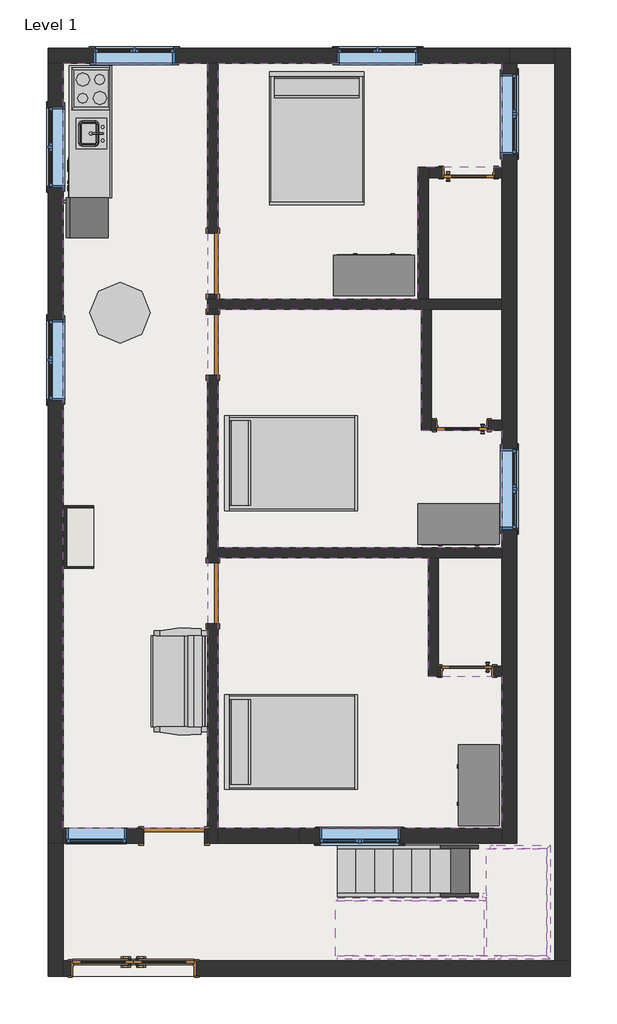
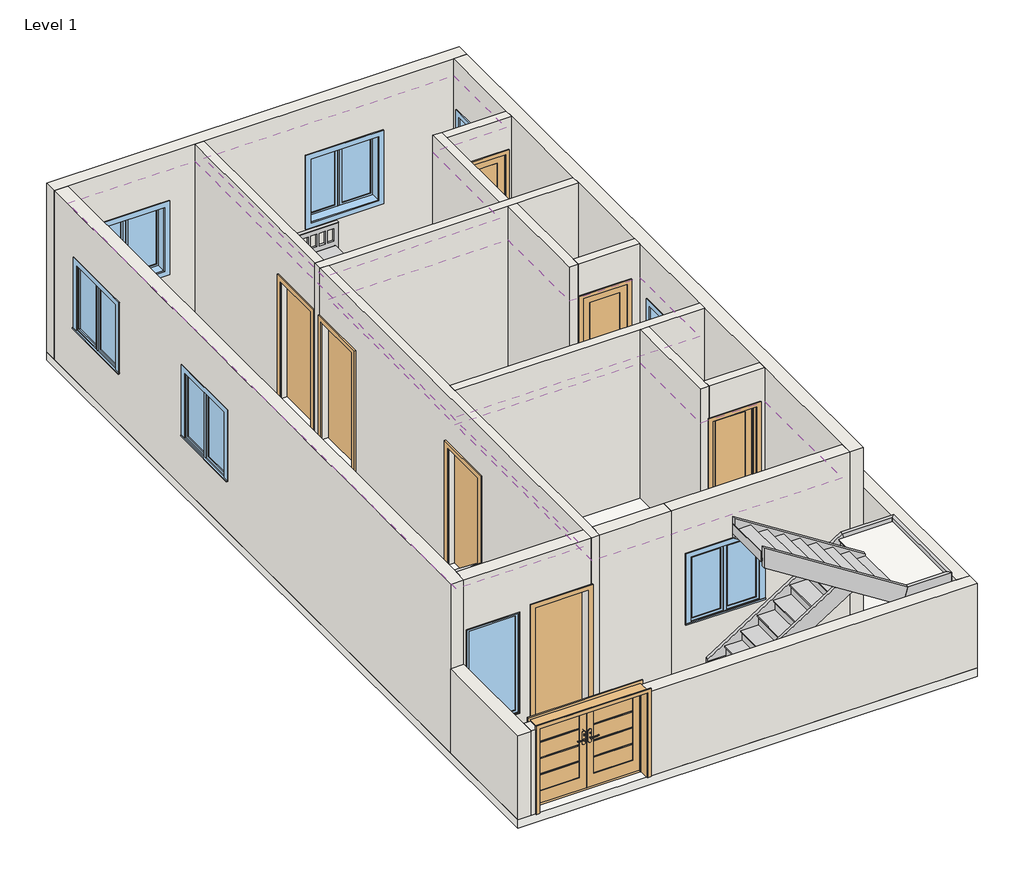
# One storey, incomplete: 21 walls, 9 furniture elements, 8 doors, 8 members, 8 windows, 4 coverings, 4 proxies, 2 slabs, 3 other elements.
"""IFC4 building model written with IfcOpenShell, lengths in millimetres."""

from ifc_helpers import new_model, si_unit, frame, origin, origin_with_axes, place, context, project, spatial, polyline, outline, extrude, faceted_brep, transform, mapped, element, save
from components import proxy_a6faaae8, proxy_45b28599, kitchenette_medium_kitchenette_medium_844211aa, proxy_c523a7b7, door_22584d03, m_door_interior_single_1_panel_wood_750_x_2400mm_65023cff, m_door_interior_single_1_panel_wood_750_x_2400mm_f8366a1a, door_16372e1c, door_686f89d2, door_0ca8825f, flow_terminal_871c2e40, furniture_096e7f55, furniture_c6510c7c, m_dresser_1220_x_1830_x_0610mm_7cb11019, m_sofa_pensi_2134mm_8f487940, furniture_905aceb5, non_monolithic_landing_dc928896, stair_flight_99ccf548, stair_flight_c84ce1c3, walls_1_walls_1_a7120c5c, window_534dcd48, window_c796fc87

model = new_model("IFC4")

# Units and contexts
model_context = context("Model", 3, world=origin())
ifc_project = project(units=[si_unit("LENGTHUNIT", "METRE", prefix="MILLI")], contexts=[model_context])

# Site, building, storey
site = spatial("IfcSite", under=ifc_project)
building = spatial("IfcBuilding", under=site)
storey = spatial("IfcBuildingStorey", under=building, Name="Level 1", Elevation=0.0)

# Proxies
placement = place(None, origin())
proxy_shape = proxy_a6faaae8(model_context)
element("IfcBuildingElementProxy", 1, Name="Cook Top-4 Unit2 : 22\" x 20\"", ObjectType="Cook Top-4 Unit2 : 22\" x 20\"", at=placement, inside=storey, context=model_context, shape_type="MappedRepresentation", body=[
    mapped(proxy_shape, transform((-8890.693556, 5030.6122215, 0.0), x_axis=(0.0, -1.0000000000000002, 0.0), y_axis=(1.0000000000000002, 0.0, 0.0), z_axis=(0.0, 0.0, 1.0))),
])
proxy_2_shape = proxy_45b28599(model_context)
element("IfcBuildingElementProxy", 2, Name="Dishwasher : 24\" x 24\" x 34\"", ObjectType="Dishwasher : 24\" x 24\" x 34\"", at=placement, inside=storey, context=model_context, shape_type="MappedRepresentation", body=[
    mapped(proxy_2_shape, transform((-9182.5431208, 4079.42969, 0.0), x_axis=(0.0, -1.0000000000000002, 0.0), y_axis=(1.0000000000000002, 0.0, 0.0), z_axis=(0.0, 0.0, 1.0))),
])
kitchenette_medium_kitchenette_medium_shape = kitchenette_medium_kitchenette_medium_844211aa(model_context)
element("IfcBuildingElementProxy", 3, Name="Kitchenette - Medium : Kitchenette - Medium", ObjectType="Kitchenette - Medium : Kitchenette - Medium", at=placement, inside=storey, context=model_context, shape_type="MappedRepresentation", body=[
    mapped(kitchenette_medium_kitchenette_medium_shape, transform((-8585.893556, 4706.4499264, 0.0), x_axis=(0.0, -1.0000000000000002, 0.0), y_axis=(1.0000000000000002, 0.0, 0.0), z_axis=(0.0, 0.0, 1.0))),
])
proxy_3_shape = proxy_c523a7b7(model_context)
element("IfcBuildingElementProxy", 4, Name="Refrigerator : 24\" x 25\" LH", ObjectType="Refrigerator : 24\" x 25\" LH", at=placement, inside=storey, context=model_context, shape_type="MappedRepresentation", body=[
    mapped(proxy_3_shape, transform((-8936.3425275, 3093.8622215, 0.0), x_axis=(0.0, -1.0000000000000002, 0.0), y_axis=(1.0000000000000002, 0.0, 0.0), z_axis=(0.0, 0.0, 1.0))),
])

# Coverings
element("IfcCovering", 5, ObjectType="2' x 4' ACT System", at=placement, inside=storey, context=model_context, shape_type="SweptSolid", body=[
    extrude(outline(polyline([(-6985.693556, 5411.6122215), (-2718.493556, 5411.6122215), (-2718.493556, 3849.5122215), (-3975.793556, 3849.5122215), (-3975.793556, 1868.3122215), (-6985.693556, 1868.3122215), (-6985.693556, 5411.6122215)])), frame((0.0, 0.0, 2743.2), z_axis=(0.0, 0.0, 1.0), x_axis=(1.0, 0.0, 0.0)), (0.0, 0.0, 1.0), 57.15),
])
element("IfcCovering", 6, ObjectType="2' x 4' ACT System", at=placement, inside=storey, context=model_context, shape_type="SweptSolid", body=[
    extrude(outline(polyline([(-2718.493556, -100.8261227), (-2718.493556, -1865.4877785), (-6985.693556, -1865.4877785), (-6985.693556, 1715.9122215), (-3925.6918655, 1715.9122215), (-3925.6918655, -100.8261227), (-2718.493556, -100.8261227)])), frame((0.0, 0.0, 2438.4), z_axis=(0.0, 0.0, 1.0), x_axis=(1.0, 0.0, 0.0)), (0.0, 0.0, 1.0), 57.15),
])
element("IfcCovering", 7, ObjectType="2' x 4' ACT System", at=placement, inside=storey, context=model_context, shape_type="SweptSolid", body=[
    extrude(outline(polyline([(-2718.493556, -3795.8877785), (-2718.493556, -6081.8877785), (-5766.493556, -6081.8877785), (-6985.693556, -6081.8877785), (-6985.693556, -2017.8877785), (-3823.393556, -2017.8877785), (-3823.393556, -3795.8877785), (-2718.493556, -3795.8877785)])), frame((0.0, 0.0, 2438.4), z_axis=(0.0, 0.0, 1.0), x_axis=(1.0, 0.0, 0.0)), (0.0, 0.0, 1.0), 57.15),
])
element("IfcCovering", 8, ObjectType="2' x 4' ACT System", at=placement, inside=storey, context=model_context, shape_type="SweptSolid", body=[
    extrude(outline(polyline([(-9309.793556, 5411.6122215), (-7138.093556, 5411.6122215), (-7138.093556, 1792.1122215), (-7138.093556, -6081.8877785), (-9309.793556, -6081.8877785), (-9309.793556, 5411.6122215)])), frame((0.0, 0.0, 2743.2), z_axis=(0.0, 0.0, 1.0), x_axis=(1.0, 0.0, 0.0)), (0.0, 0.0, 1.0), 57.15),
])

# Doors
door_shape = door_22584d03(model_context)
element("IfcDoor", 9, ObjectType="Door-Exterior-Double-Full Glass-Wood_Clad : 72\" x 60\"", at=placement, inside=storey, context=model_context, shape_type="MappedRepresentation", body=[
    mapped(door_shape, transform((-8255.693556, -8186.9127785, 0.0), x_axis=(1.0, 0.0, 0.0), y_axis=(0.0, 1.0, 0.0), z_axis=(0.0, 0.0, 1.0))),
])
m_door_interior_single_1_panel_wood_750_x_2400mm_shape = m_door_interior_single_1_panel_wood_750_x_2400mm_65023cff(model_context)
element("IfcDoor", 10, ObjectType="M_Door-Interior-Single-1_Panel-Wood : 750 x 2400mm", at=placement, inside=storey, context=model_context, shape_type="MappedRepresentation", body=[
    mapped(m_door_interior_single_1_panel_wood_750_x_2400mm_shape, transform((-3213.793556, 3770.1372215, 0.0), x_axis=(1.0, 0.0, 0.0), y_axis=(0.0, 1.0, 0.0), z_axis=(0.0, 0.0, 1.0))),
])
element("IfcDoor", 11, ObjectType="M_Door-Interior-Single-1_Panel-Wood : 750 x 2400mm", at=placement, inside=storey, context=model_context, shape_type="MappedRepresentation", body=[
    mapped(m_door_interior_single_1_panel_wood_750_x_2400mm_shape, transform((-3239.193556, -3716.5127785, 0.0), x_axis=(-1.0, 0.0, 0.0), y_axis=(0.0, -1.0, 0.0), z_axis=(0.0, 0.0, 1.0))),
])
m_door_interior_single_1_panel_wood_750_x_2400mm_2_shape = m_door_interior_single_1_panel_wood_750_x_2400mm_f8366a1a(model_context)
element("IfcDoor", 12, ObjectType="M_Door-Interior-Single-1_Panel-Wood : 750 x 2400mm", at=placement, inside=storey, context=model_context, shape_type="MappedRepresentation", body=[
    mapped(m_door_interior_single_1_panel_wood_750_x_2400mm_2_shape, transform((-3316.0918655, -27.8011227, 0.0), x_axis=(-1.0, 0.0, 0.0), y_axis=(0.0, -1.0, 0.0), z_axis=(0.0, 0.0, 1.0))),
])
door_2_shape = door_16372e1c(model_context)
element("IfcDoor", 13, ObjectType="Single-Flush : 36\" x 84\"", at=placement, inside=storey, context=model_context, shape_type="MappedRepresentation", body=[
    mapped(door_2_shape, transform((-7061.893556, 2401.7122215, 0.0), x_axis=(0.0, -1.0, 0.0), y_axis=(1.0, 0.0, 0.0), z_axis=(0.0, 0.0, 1.0))),
])
door_3_shape = door_686f89d2(model_context)
element("IfcDoor", 14, ObjectType="Single-Flush : 36\" x 84\"", at=placement, inside=storey, context=model_context, shape_type="MappedRepresentation", body=[
    mapped(door_3_shape, transform((-7061.893556, 1182.5122215, 0.0), x_axis=(0.0, 1.0, 0.0), y_axis=(-1.0, 0.0, 0.0), z_axis=(0.0, 0.0, 1.0))),
])
element("IfcDoor", 15, ObjectType="Single-Flush : 36\" x 84\"", at=placement, inside=storey, context=model_context, shape_type="MappedRepresentation", body=[
    mapped(door_3_shape, transform((-7061.893556, -2551.2877785, 0.0), x_axis=(0.0, 1.0, 0.0), y_axis=(-1.0, 0.0, 0.0), z_axis=(0.0, 0.0, 1.0))),
])
door_4_shape = door_0ca8825f(model_context)
element("IfcDoor", 16, ObjectType="Single-Flush : 36\" x 84\"", at=placement, inside=storey, context=model_context, shape_type="MappedRepresentation", body=[
    mapped(door_4_shape, transform((-7646.093556, -6196.1877785, 0.0), x_axis=(1.0, 0.0, 0.0), y_axis=(0.0, 1.0, 0.0), z_axis=(0.0, 0.0, 1.0))),
])

# Flow terminal
flow_terminal_shape = flow_terminal_871c2e40(model_context)
element("IfcFlowTerminal", 17, ObjectType="Sink Kitchen-Island : 18\" x 18\"", at=placement, inside=storey, context=model_context, shape_type="MappedRepresentation", body=[
    mapped(flow_terminal_shape, transform((-8893.0389571, 4373.2014621, -14.4), x_axis=(0.0, -1.0000000000000002, 0.0), y_axis=(1.0000000000000002, 0.0, 0.0), z_axis=(0.0, 0.0, 1.0))),
])

# Furniture
furniture_shape = furniture_096e7f55(model_context)
element("IfcFurniture", 18, ObjectType="Bed-Shaker : Double 56\" x 78\"", at=placement, inside=storey, context=model_context, shape_type="MappedRepresentation", body=[
    mapped(furniture_shape, transform((-5480.743556, 5271.9122215, 0.0), x_axis=(1.0, 0.0, 0.0), y_axis=(0.0, 1.0, 0.0), z_axis=(0.0, 0.0, 1.0))),
])
element("IfcFurniture", 19, ObjectType="Bed-Shaker : Double 56\" x 78\"", at=placement, inside=storey, context=model_context, shape_type="MappedRepresentation", body=[
    mapped(furniture_shape, transform((-6871.393556, -576.4377785, 0.0), x_axis=(0.0, 1.0000000000000004, 0.0), y_axis=(-1.0000000000000004, 0.0, 0.0), z_axis=(0.0, 0.0, 1.0))),
])
element("IfcFurniture", 20, ObjectType="Bed-Shaker : Double 56\" x 78\"", at=placement, inside=storey, context=model_context, shape_type="MappedRepresentation", body=[
    mapped(furniture_shape, transform((-6871.393556, -4767.4377785, 0.0), x_axis=(0.0, 1.0, 0.0), y_axis=(-1.0, 0.0, 0.0), z_axis=(0.0, 0.0, 1.0))),
])
furniture_2_shape = furniture_c6510c7c(model_context)
element("IfcFurniture", 21, ObjectType="Counter Top w Sink Hole : 24\" Depth", at=placement, inside=storey, context=model_context, shape_type="MappedRepresentation", body=[
    mapped(furniture_2_shape, transform((-8585.893556, 4173.0499264, -14.4), x_axis=(0.0, -1.0000000000000002, 0.0), y_axis=(1.0000000000000002, 0.0, 0.0), z_axis=(0.0, 0.0, 1.0))),
])
m_dresser_1220_x_1830_x_0610mm_shape = m_dresser_1220_x_1830_x_0610mm_7cb11019(model_context)
element("IfcFurniture", 22, ObjectType="M_Dresser : 1220 x 1830 x 0610mm", at=placement, inside=storey, context=model_context, shape_type="MappedRepresentation", body=[
    mapped(m_dresser_1220_x_1830_x_0610mm_shape, transform((-3096.8002962, -1147.1248244, 0.0), x_axis=(1.0000000000000009, 0.0, 0.0), y_axis=(0.0, 1.0000000000000009, 0.0), z_axis=(0.0, 0.0, 1.0))),
])
element("IfcFurniture", 23, ObjectType="M_Dresser : 1220 x 1830 x 0610mm", at=placement, inside=storey, context=model_context, shape_type="MappedRepresentation", body=[
    mapped(m_dresser_1220_x_1830_x_0610mm_shape, transform((-4908.0117472, 1860.9492674, 0.0), x_axis=(-1.0000000000000009, 0.0, 0.0), y_axis=(0.0, -1.0000000000000009, 0.0), z_axis=(0.0, 0.0, 1.0))),
])
element("IfcFurniture", 24, ObjectType="M_Dresser : 1220 x 1830 x 0610mm", at=placement, inside=storey, context=model_context, shape_type="MappedRepresentation", body=[
    mapped(m_dresser_1220_x_1830_x_0610mm_shape, transform((-2698.4306019, -5702.9810383, 0.0), x_axis=(0.0, -1.0, 0.0), y_axis=(1.0, 0.0, 0.0), z_axis=(0.0, 0.0, 1.0))),
])
m_sofa_pensi_2134mm_shape = m_sofa_pensi_2134mm_8f487940(model_context)
element("IfcFurniture", 25, ObjectType="M_Sofa-Pensi : 2134mm", at=placement, inside=storey, context=model_context, shape_type="MappedRepresentation", body=[
    mapped(m_sofa_pensi_2134mm_shape, transform((-7847.0033921, -3593.4815285, 0.0), x_axis=(0.0, -1.0000000000000002, 0.0), y_axis=(1.0000000000000002, 0.0, 0.0), z_axis=(0.0, 0.0, 1.0))),
])
furniture_3_shape = furniture_905aceb5(model_context)
element("IfcFurniture", 26, ObjectType="Table-Dining Round w Chairs : 36\" Diameter", at=placement, inside=storey, context=model_context, shape_type="MappedRepresentation", body=[
    mapped(furniture_3_shape, transform((-8562.5755232, 1849.99091, 0.0), x_axis=(1.0, 0.0, 0.0), y_axis=(0.0, 1.0, 0.0), z_axis=(0.0, 0.0, 1.0))),
])

# Members
element("IfcMember", 27, ObjectType="Stringer - 2\" Width", at=placement, inside=storey, context=model_context, shape_type="SweptSolid", body=[
    extrude(outline(polyline([(215.0106437, -5185.8837185), (0.0, -5185.8837185), (0.0, -4956.0281891), (1371.6, -2800.6567606), (1676.4, -2889.41473), (215.0106437, -5185.8837185)])), frame((0.0, -6386.6877785, 0.0), z_axis=(0.0, 1.0, 0.0), x_axis=(0.0, 0.0, 1.0)), (0.0, 0.0, 1.0), 50.8),
])
element("IfcMember", 28, ObjectType="Stringer - 2\" Width", at=placement, inside=storey, context=model_context, shape_type="SweptSolid", body=[
    extrude(outline(polyline([(215.0106437, -5185.8837185), (0.0, -5185.8837185), (0.0, -4956.0281891), (1243.8010268, -3001.4837185), (1605.083371, -3001.4837185), (215.0106437, -5185.8837185)])), frame((0.0, -7111.7366292, 0.0), z_axis=(0.0, 1.0, 0.0), x_axis=(0.0, 0.0, 1.0)), (0.0, 0.0, 1.0), 50.8),
])
element("IfcMember", 29, ObjectType="Stringer - 2\" Width", at=placement, inside=storey, context=model_context, shape_type="SweptSolid", body=[
    extrude(outline(polyline([(1371.6, -2821.3106764), (1676.4, -2732.552707), (3237.6106437, -5185.8837185), (2876.3282995, -5185.8837185), (1371.6, -2821.3106764)])), frame((0.0, -8051.5366292, 0.0), z_axis=(0.0, 1.0, 0.0), x_axis=(0.0, 0.0, 1.0)), (0.0, 0.0, 1.0), 50.8),
])
element("IfcMember", 30, ObjectType="Stringer - 2\" Width", at=placement, inside=storey, context=model_context, shape_type="SweptSolid", body=[
    extrude(outline(polyline([(1453.9282995, -2950.6837185), (1815.2106437, -2950.6837185), (3237.6106437, -5185.8837185), (2876.3282995, -5185.8837185), (1453.9282995, -2950.6837185)])), frame((0.0, -7174.0877785, 0.0), z_axis=(0.0, 1.0, 0.0), x_axis=(0.0, 0.0, 1.0)), (0.0, 0.0, 1.0), 50.8),
])
element("IfcMember", 31, ObjectType="Stringer - 2\" Width", at=placement, inside=storey, context=model_context, shape_type="Brep", body=[
    faceted_brep([(-2732.552707, -8000.7366292, 1676.4), (-2732.552707, -8051.5366292, 1676.4), (-1985.4837185, -8051.5366292, 1676.4), (-2036.2837185, -8000.7366292, 1676.4), (-2821.3106764, -8000.7366292, 1371.6), (-2036.2837185, -8000.7366292, 1371.6), (-2821.3106764, -8051.5366292, 1371.6), (-1985.4837185, -8051.5366292, 1371.6)], [[[0, 1, 2, 3]], [[4, 0, 3, 5]], [[6, 4, 5, 7]], [[1, 6, 7, 2]], [[1, 0, 4, 6]], [[2, 7, 5, 3]]]),
])
element("IfcMember", 32, ObjectType="Stringer - 2\" Width", at=placement, inside=storey, context=model_context, shape_type="SweptSolid", body=[
    extrude(outline(polyline([(-1985.4837185, -8051.5366292), (-2036.2837185, -8000.7366292), (-2036.2837185, -6386.6877785), (-1985.4837185, -6335.8877785), (-1985.4837185, -8051.5366292)])), frame((0.0, 0.0, 1371.6), z_axis=(0.0, 0.0, 1.0), x_axis=(1.0, 0.0, 0.0)), (0.0, 0.0, 1.0), 304.8),
])
element("IfcMember", 33, ObjectType="Stringer - 2\" Width", at=placement, inside=storey, context=model_context, shape_type="Brep", body=[
    faceted_brep([(-2036.2837185, -6386.6877785, 1676.4), (-1985.4837185, -6335.8877785, 1676.4), (-2889.41473, -6335.8877785, 1676.4), (-2889.41473, -6386.6877785, 1676.4), (-2036.2837185, -6386.6877785, 1371.6), (-2800.6567606, -6386.6877785, 1371.6), (-1985.4837185, -6335.8877785, 1371.6), (-2800.6567606, -6335.8877785, 1371.6)], [[[0, 1, 2, 3]], [[4, 0, 3, 5]], [[6, 4, 5, 7]], [[1, 6, 7, 2]], [[1, 0, 4, 6]], [[2, 7, 5, 3]]]),
])
element("IfcMember", 34, ObjectType="Stringer - 2\" Width", at=placement, inside=storey, context=model_context, shape_type="SweptSolid", body=[
    extrude(outline(polyline([(-3001.4837185, -7060.9366292), (-2950.6837185, -7060.9366292), (-2950.6837185, -7123.2877785), (-3001.4837185, -7123.2877785), (-3001.4837185, -7060.9366292)])), frame((0.0, 0.0, 1371.6), z_axis=(0.0, 0.0, 1.0), x_axis=(1.0, 0.0, 0.0)), (0.0, 0.0, 1.0), 304.8),
])

# Slabs
element("IfcSlab", 35, ObjectType="6\"", at=placement, inside=storey, context=model_context, shape_type="SweptSolid", body=[
    extrude(outline(polyline([(-1689.793556, 5640.2122215), (-1689.793556, -8304.3877785), (-9538.393556, -8304.3877785), (-9538.393556, 5640.2122215), (-1689.793556, 5640.2122215)])), frame((0.0, 0.0, -152.4), z_axis=(0.0, 0.0, 1.0), x_axis=(1.0, 0.0, 0.0)), (0.0, 0.0, 1.0), 152.4),
])
non_monolithic_landing_shape = non_monolithic_landing_dc928896(model_context)
element("IfcSlab", 36, ObjectType="Non-Monolithic Landing", at=placement, inside=storey, context=model_context, shape_type="MappedRepresentation", body=[
    mapped(non_monolithic_landing_shape, transform((0.0, 0.0, 0.0), x_axis=(1.0, 0.0, 0.0), y_axis=(0.0, 1.0, 0.0), z_axis=(0.0, 0.0, 1.0))),
])

# Stair flights
stair_flight_shape = stair_flight_99ccf548(model_context)
element("IfcStairFlight", 37, ObjectType="2\" Tread 1\" Nosing 1/4\" Riser", at=placement, inside=storey, context=model_context, shape_type="MappedRepresentation", body=[
    mapped(stair_flight_shape, transform((0.0, 0.0, 0.0), x_axis=(1.0, 0.0, 0.0), y_axis=(0.0, 1.0, 0.0), z_axis=(0.0, 0.0, 1.0))),
])
stair_flight_2_shape = stair_flight_c84ce1c3(model_context)
element("IfcStairFlight", 38, ObjectType="2\" Tread 1\" Nosing 1/4\" Riser", at=placement, inside=storey, context=model_context, shape_type="MappedRepresentation", body=[
    mapped(stair_flight_2_shape, transform((0.0, 0.0, 0.0), x_axis=(1.0, 0.0, 0.0), y_axis=(0.0, 1.0, 0.0), z_axis=(0.0, 0.0, 1.0))),
])

# Walls
element("IfcWall", 39, ObjectType="6\"", at=placement, inside=storey, context=model_context, shape_type="Brep", body=[
    faceted_brep([(-2718.493556, 1868.3122215, 0.0), (-3823.393556, 1868.3122215, 0.0), (-3975.793556, 1868.3122215, 0.0), (-6985.693556, 1868.3122215, 0.0), (-7138.093556, 1868.3122215, 0.0), (-7138.093556, 1868.3122215, 3048.0), (-6985.693556, 1868.3122215, 3048.0), (-3975.793556, 1868.3122215, 3048.0), (-3823.393556, 1868.3122215, 3048.0), (-2718.493556, 1868.3122215, 3048.0), (-2718.493556, 1715.9122215, 0.0), (-2718.493556, 1715.9122215, 3048.0), (-3773.2918655, 1715.9122215, 3048.0), (-3925.6918655, 1715.9122215, 3048.0), (-6985.693556, 1715.9122215, 3048.0), (-7138.093556, 1715.9122215, 3048.0), (-7138.093556, 1715.9122215, 0.0), (-6985.693556, 1715.9122215, 0.0), (-3925.6918655, 1715.9122215, 0.0), (-3773.2918655, 1715.9122215, 0.0)], [[[0, 1, 2, 3, 4, 5, 6, 7, 8, 9]], [[10, 11, 12, 13, 14, 15, 16, 17, 18, 19]], [[4, 3, 2, 1, 0, 10, 19, 18, 17, 16]], [[9, 8, 7, 6, 5, 15, 14, 13, 12, 11]], [[0, 9, 11, 10]], [[5, 4, 16, 15]]]),
])
element("IfcWall", 40, ObjectType="6\"", at=placement, inside=storey, context=model_context, shape_type="SweptSolid", body=[
    extrude(outline(polyline([(1944.5122215, 2133.6), (1944.5122215, 0.0), (1868.3122215, 0.0), (1868.3122215, 3048.0), (5411.6122215, 3048.0), (5411.6122215, 0.0), (2858.9122215, 0.0), (2858.9122215, 2133.6), (1944.5122215, 2133.6)])), frame((-7138.093556, 0.0, 0.0), z_axis=(1.0, 0.0, 0.0), x_axis=(0.0, 1.0, 0.0)), (0.0, 0.0, 1.0), 152.4),
])
element("IfcWall", 41, ObjectType="6\"", at=placement, inside=storey, context=model_context, shape_type="Brep", body=[
    faceted_brep([(-3823.393556, 1868.3122215, 0.0), (-3823.393556, 3697.1122215, 0.0), (-3823.393556, 3849.5122215, 0.0), (-3823.393556, 3849.5122215, 3048.0), (-3823.393556, 3697.1122215, 3048.0), (-3823.393556, 1868.3122215, 3048.0), (-3975.793556, 1868.3122215, 0.0), (-3975.793556, 1868.3122215, 3048.0), (-3975.793556, 3849.5122215, 3048.0), (-3975.793556, 3849.5122215, 0.0)], [[[0, 1, 2, 3, 4, 5]], [[6, 7, 8, 9]], [[2, 1, 0, 6, 9]], [[5, 4, 3, 8, 7]], [[0, 5, 7, 6]], [[3, 2, 9, 8]]]),
])
element("IfcWall", 42, ObjectType="6\"", at=placement, inside=storey, context=model_context, shape_type="SweptSolid", body=[
    extrude(outline(polyline([(3048.0, -2718.493556), (3048.0, -3823.393556), (0.0, -3823.393556), (0.0, -3613.793556), (2425.0, -3613.793556), (2425.0, -2813.793556), (0.0, -2813.793556), (0.0, -2718.493556), (3048.0, -2718.493556)])), frame((0.0, 3697.1122215, 0.0), z_axis=(0.0, 1.0, 0.0), x_axis=(0.0, 0.0, 1.0)), (0.0, 0.0, 1.0), 152.4),
])
element("IfcWall", 43, ObjectType="6\"", at=placement, inside=storey, context=model_context, shape_type="Brep", body=[
    faceted_brep([(-2718.493556, -1865.4877785, 0.0), (-6985.693556, -1865.4877785, 0.0), (-6985.693556, -1865.4877785, 3048.0), (-2718.493556, -1865.4877785, 3048.0), (-2718.493556, -2017.8877785, 0.0), (-2718.493556, -2017.8877785, 3048.0), (-3670.993556, -2017.8877785, 3048.0), (-3823.393556, -2017.8877785, 3048.0), (-6985.693556, -2017.8877785, 3048.0), (-6985.693556, -2017.8877785, 0.0), (-3823.393556, -2017.8877785, 0.0), (-3670.993556, -2017.8877785, 0.0)], [[[0, 1, 2, 3]], [[4, 5, 6, 7, 8, 9, 10, 11]], [[1, 0, 4, 11, 10, 9]], [[3, 2, 8, 7, 6, 5]], [[0, 3, 5, 4]], [[2, 1, 9, 8]]]),
])
element("IfcWall", 44, ObjectType="6\"", at=placement, inside=storey, context=model_context, shape_type="Brep", body=[
    faceted_brep([(-7138.093556, 725.3122215, 0.0), (-7138.093556, -2094.0877785, 0.0), (-7138.093556, -2094.0877785, 2133.6), (-7138.093556, -3008.4877785, 2133.6), (-7138.093556, -3008.4877785, 0.0), (-7138.093556, -6081.8877785, 0.0), (-7138.093556, -6310.4877785, 0.0), (-7138.093556, -6310.4877785, 3048.0), (-7138.093556, -6081.8877785, 3048.0), (-7138.093556, 1715.9122215, 3048.0), (-7138.093556, 1715.9122215, 0.0), (-7138.093556, 1639.7122215, 0.0), (-7138.093556, 1639.7122215, 2133.6), (-7138.093556, 725.3122215, 2133.6), (-6985.693556, -2094.0877785, 2133.6), (-6985.693556, -2094.0877785, 0.0), (-6985.693556, -2017.8877785, 0.0), (-6985.693556, -1865.4877785, 0.0), (-6985.693556, 725.3122215, 0.0), (-6985.693556, 725.3122215, 2133.6), (-6985.693556, 1639.7122215, 2133.6), (-6985.693556, 1639.7122215, 0.0), (-6985.693556, 1715.9122215, 0.0), (-6985.693556, 1715.9122215, 3048.0), (-6985.693556, -1865.4877785, 3048.0), (-6985.693556, -2017.8877785, 3048.0), (-6985.693556, -6081.8877785, 3048.0), (-6985.693556, -6310.4877785, 3048.0), (-6985.693556, -6310.4877785, 0.0), (-6985.693556, -6081.8877785, 0.0), (-6985.693556, -3008.4877785, 0.0), (-6985.693556, -3008.4877785, 2133.6)], [[[0, 1, 2, 3, 4, 5, 6, 7, 8, 9, 10, 11, 12, 13]], [[14, 15, 16, 17, 18, 19, 20, 21, 22, 23, 24, 25, 26, 27, 28, 29, 30, 31]], [[22, 21, 11, 10]], [[30, 29, 28, 6, 5, 4]], [[18, 17, 16, 15, 1, 0]], [[9, 8, 7, 27, 26, 25, 24, 23]], [[10, 9, 23, 22]], [[7, 6, 28, 27]], [[12, 11, 21, 20]], [[13, 12, 20, 19]], [[0, 13, 19, 18]], [[2, 1, 15, 14]], [[3, 2, 14, 31]], [[4, 3, 31, 30]]]),
])
element("IfcWall", 45, ObjectType="6\"", at=placement, inside=storey, context=model_context, shape_type="Brep", body=[
    faceted_brep([(-3823.393556, -2017.8877785, 0.0), (-3823.393556, -3795.8877785, 0.0), (-3823.393556, -3795.8877785, 3048.0), (-3823.393556, -2017.8877785, 3048.0), (-3670.993556, -2017.8877785, 0.0), (-3670.993556, -2017.8877785, 3048.0), (-3670.993556, -3643.4877785, 3048.0), (-3670.993556, -3795.8877785, 3048.0), (-3670.993556, -3795.8877785, 0.0), (-3670.993556, -3643.4877785, 0.0)], [[[0, 1, 2, 3]], [[4, 5, 6, 7, 8, 9]], [[1, 0, 4, 9, 8]], [[3, 2, 7, 6, 5]], [[0, 3, 5, 4]], [[2, 1, 8, 7]]]),
])
element("IfcWall", 46, ObjectType="6\"", at=placement, inside=storey, context=model_context, shape_type="SweptSolid", body=[
    extrude(outline(polyline([(3048.0, -2718.493556), (3048.0, -3670.993556), (0.0, -3670.993556), (0.0, -3639.193556), (2425.0, -3639.193556), (2425.0, -2839.193556), (0.0, -2839.193556), (0.0, -2718.493556), (3048.0, -2718.493556)])), frame((0.0, -3795.8877785, 0.0), z_axis=(0.0, 1.0, 0.0), x_axis=(0.0, 0.0, 1.0)), (0.0, 0.0, 1.0), 152.4),
])
element("IfcWall", 47, ObjectType="6\"", at=placement, inside=storey, context=model_context, shape_type="Brep", body=[
    faceted_brep([(-3925.6918655, 1715.9122215, 0.0), (-3925.6918655, -100.8261227, 0.0), (-3925.6918655, -100.8261227, 3048.0), (-3925.6918655, 1715.9122215, 3048.0), (-3773.2918655, 1715.9122215, 0.0), (-3773.2918655, 1715.9122215, 3048.0), (-3773.2918655, 51.5738773, 3048.0), (-3773.2918655, -100.8261227, 3048.0), (-3773.2918655, -100.8261227, 0.0), (-3773.2918655, 51.5738773, 0.0)], [[[0, 1, 2, 3]], [[4, 5, 6, 7, 8, 9]], [[1, 0, 4, 9, 8]], [[3, 2, 7, 6, 5]], [[2, 1, 8, 7]], [[0, 3, 5, 4]]]),
])
element("IfcWall", 48, ObjectType="6\"", at=placement, inside=storey, context=model_context, shape_type="SweptSolid", body=[
    extrude(outline(polyline([(3048.0, -2718.493556), (3048.0, -3773.2918655), (0.0, -3773.2918655), (0.0, -3716.0918655), (2425.0, -3716.0918655), (2425.0, -2916.0918655), (0.0, -2916.0918655), (0.0, -2718.493556), (3048.0, -2718.493556)])), frame((0.0, -100.8261227, 0.0), z_axis=(0.0, 1.0, 0.0), x_axis=(0.0, 0.0, 1.0)), (0.0, 0.0, 1.0), 152.4),
])
element("IfcWall", 49, ObjectType="9\"", at=placement, inside=storey, context=model_context, shape_type="Brep", body=[
    faceted_brep([(-9538.393556, 5411.6122215, 0.0), (-9309.793556, 5411.6122215, 0.0), (-7138.093556, 5411.6122215, 0.0), (-6985.693556, 5411.6122215, 0.0), (-2718.493556, 5411.6122215, 0.0), (-2604.193556, 5411.6122215, 0.0), (-2604.193556, 5411.6122215, 1539.3845055), (-2489.893556, 5411.6122215, 1539.3845055), (-2489.893556, 5411.6122215, 3048.0), (-2718.493556, 5411.6122215, 3048.0), (-6985.693556, 5411.6122215, 3048.0), (-7138.093556, 5411.6122215, 3048.0), (-9309.793556, 5411.6122215, 3048.0), (-9538.393556, 5411.6122215, 3048.0), (-3975.793556, 5411.6122215, 2133.6), (-3975.793556, 5411.6122215, 914.4), (-5194.993556, 5411.6122215, 914.4), (-5194.993556, 5411.6122215, 2133.6), (-7633.393556, 5411.6122215, 2133.6), (-7633.393556, 5411.6122215, 914.4), (-8852.593556, 5411.6122215, 914.4), (-8852.593556, 5411.6122215, 2133.6), (-9538.393556, 5640.2122215, 0.0), (-9538.393556, 5640.2122215, 3048.0), (-2489.893556, 5640.2122215, 3048.0), (-2489.893556, 5640.2122215, 1539.3845055), (-2604.193556, 5640.2122215, 1539.3845055), (-2604.193556, 5640.2122215, 0.0), (-3975.793556, 5640.2122215, 2133.6), (-5194.993556, 5640.2122215, 2133.6), (-5194.993556, 5640.2122215, 914.4), (-3975.793556, 5640.2122215, 914.4), (-7633.393556, 5640.2122215, 2133.6), (-8852.593556, 5640.2122215, 2133.6), (-8852.593556, 5640.2122215, 914.4), (-7633.393556, 5640.2122215, 914.4)], [[[0, 1, 2, 3, 4, 5, 6, 7, 8, 9, 10, 11, 12, 13], [14, 15, 16, 17], [18, 19, 20, 21]], [[22, 23, 24, 25, 26, 27], [28, 29, 30, 31], [32, 33, 34, 35]], [[5, 4, 3, 2, 1, 0, 22, 27]], [[13, 12, 11, 10, 9, 8, 24, 23]], [[0, 13, 23, 22]], [[6, 5, 27, 26]], [[25, 7, 6, 26]], [[8, 7, 25, 24]], [[15, 14, 28, 31]], [[16, 15, 31, 30]], [[17, 16, 30, 29]], [[14, 17, 29, 28]], [[19, 18, 32, 35]], [[20, 19, 35, 34]], [[21, 20, 34, 33]], [[18, 21, 33, 32]]]),
])
element("IfcWall", 50, ObjectType="9\"", at=placement, inside=storey, context=model_context, shape_type="Brep", body=[
    faceted_brep([(-9309.793556, -8304.3877785, 0.0), (-9309.793556, -8075.7877785, 0.0), (-9309.793556, -6310.4877785, 0.0), (-9309.793556, -6310.4877785, 1522.2082431), (-9309.793556, -8304.3877785, 1522.2082431), (-9538.393556, -8304.3877785, 0.0), (-9538.393556, -8304.3877785, 1522.2082431), (-9538.393556, -6310.4877785, 1522.2082431), (-9538.393556, -6310.4877785, 0.0)], [[[0, 1, 2, 3, 4]], [[5, 6, 7, 8]], [[2, 1, 0, 5, 8]], [[3, 2, 8, 7]], [[4, 3, 7, 6]], [[0, 4, 6, 5]]]),
])
element("IfcWall", 51, ObjectType="9\"", at=placement, inside=storey, context=model_context, shape_type="Brep", body=[
    faceted_brep([(-9309.793556, -8075.7877785, 0.0), (-9309.793556, -8075.7877785, 1524.0), (-9195.493556, -8075.7877785, 1524.0), (-9195.493556, -8075.7877785, 0.0), (-9309.793556, -8304.3877785, 1524.0), (-9309.793556, -8304.3877785, 1522.2082431), (-9309.793556, -8304.3877785, 0.0), (-9195.493556, -8304.3877785, 0.0), (-9195.493556, -8304.3877785, 1524.0)], [[[0, 1, 2, 3]], [[4, 5, 6, 7, 8]], [[6, 0, 3, 7]], [[1, 4, 8, 2]], [[1, 0, 6, 5, 4]], [[3, 2, 8, 7]]]),
    faceted_brep([(-1689.793556, -8075.7877785, 1524.0), (-1689.793556, -8075.7877785, 0.0), (-1918.393556, -8075.7877785, 0.0), (-7315.893556, -8075.7877785, 0.0), (-7315.893556, -8075.7877785, 1524.0), (-1918.393556, -8075.7877785, 1524.0), (-1689.793556, -8304.3877785, 0.0), (-1689.793556, -8304.3877785, 1524.0), (-7315.893556, -8304.3877785, 1524.0), (-7315.893556, -8304.3877785, 0.0)], [[[0, 1, 2, 3, 4, 5]], [[6, 7, 8, 9]], [[1, 6, 9, 3, 2]], [[7, 0, 5, 4, 8]], [[1, 0, 7, 6]], [[4, 3, 9, 8]]]),
])
element("IfcWall", 52, ObjectType="9\"", at=placement, inside=storey, context=model_context, shape_type="Brep", body=[
    faceted_brep([(-1918.393556, 5640.2122215, 0.0), (-1918.393556, 5411.6122215, 0.0), (-1918.393556, -8075.7877785, 0.0), (-1918.393556, -8075.7877785, 1524.0), (-1918.393556, 5640.2122215, 1524.0), (-1689.793556, 5640.2122215, 0.0), (-1689.793556, 5640.2122215, 1524.0), (-1689.793556, -8075.7877785, 1524.0), (-1689.793556, -8075.7877785, 0.0)], [[[0, 1, 2, 3, 4]], [[5, 6, 7, 8]], [[2, 1, 0, 5, 8]], [[4, 3, 7, 6]], [[0, 4, 6, 5]], [[3, 2, 8, 7]]]),
])
element("IfcWall", 53, ObjectType="9\"", at=placement, inside=storey, context=model_context, shape_type="Brep", body=[
    faceted_brep([(-2718.493556, 5411.6122215, 3048.0), (-2718.493556, 5411.6122215, 0.0), (-2718.493556, 3849.5122215, 0.0), (-2718.493556, 3697.1122215, 0.0), (-2718.493556, 1868.3122215, 0.0), (-2718.493556, 1715.9122215, 0.0), (-2718.493556, 51.5738773, 0.0), (-2718.493556, -100.8261227, 0.0), (-2718.493556, -1865.4877785, 0.0), (-2718.493556, -2017.8877785, 0.0), (-2718.493556, -3643.4877785, 0.0), (-2718.493556, -3795.8877785, 0.0), (-2718.493556, -6081.8877785, 0.0), (-2718.493556, -6310.4877785, 0.0), (-2718.493556, -6310.4877785, 3048.0), (-2718.493556, -6081.8877785, 3048.0), (-2718.493556, -3795.8877785, 3048.0), (-2718.493556, -3643.4877785, 3048.0), (-2718.493556, -2017.8877785, 3048.0), (-2718.493556, -1865.4877785, 3048.0), (-2718.493556, -100.8261227, 3048.0), (-2718.493556, 51.5738773, 3048.0), (-2718.493556, 1715.9122215, 3048.0), (-2718.493556, 1868.3122215, 3048.0), (-2718.493556, 3697.1122215, 3048.0), (-2718.493556, 3849.5122215, 3048.0), (-2718.493556, -1592.7569506, 2133.6), (-2718.493556, -1592.7569506, 914.4), (-2718.493556, -373.5569506, 914.4), (-2718.493556, -373.5569506, 2133.6), (-2718.493556, 4040.0122215, 2133.6), (-2718.493556, 4040.0122215, 914.4), (-2718.493556, 5259.2122215, 914.4), (-2718.493556, 5259.2122215, 2133.6), (-2489.893556, 5411.6122215, 0.0), (-2489.893556, 5411.6122215, 1539.3845055), (-2489.893556, 5411.6122215, 3048.0), (-2489.893556, -6310.4877785, 3048.0), (-2489.893556, -6310.4877785, 0.0), (-2489.893556, -1592.7569506, 2133.6), (-2489.893556, -373.5569506, 2133.6), (-2489.893556, -373.5569506, 914.4), (-2489.893556, -1592.7569506, 914.4), (-2489.893556, 4040.0122215, 2133.6), (-2489.893556, 5259.2122215, 2133.6), (-2489.893556, 5259.2122215, 914.4), (-2489.893556, 4040.0122215, 914.4), (-2604.193556, 5411.6122215, 0.0)], [[[0, 1, 2, 3, 4, 5, 6, 7, 8, 9, 10, 11, 12, 13, 14, 15, 16, 17, 18, 19, 20, 21, 22, 23, 24, 25], [26, 27, 28, 29], [30, 31, 32, 33]], [[34, 35, 36, 37, 38], [39, 40, 41, 42], [43, 44, 45, 46]], [[13, 12, 11, 10, 9, 8, 7, 6, 5, 4, 3, 2, 1, 47, 34, 38]], [[14, 13, 38, 37]], [[0, 25, 24, 23, 22, 21, 20, 19, 18, 17, 16, 15, 14, 37, 36]], [[0, 36, 35, 34, 47, 1]], [[27, 26, 39, 42]], [[28, 27, 42, 41]], [[29, 28, 41, 40]], [[26, 29, 40, 39]], [[31, 30, 43, 46]], [[32, 31, 46, 45]], [[33, 32, 45, 44]], [[30, 33, 44, 43]]]),
])
element("IfcWall", 54, ObjectType="9\"", at=placement, inside=storey, context=model_context, shape_type="SweptSolid", body=[
    extrude(outline(polyline([(0.0, -2718.493556), (3048.0, -2718.493556), (3048.0, -5766.493556), (0.0, -5766.493556), (0.0, -2718.493556)]), holes=[polyline([(2133.6, -5461.693556), (2133.6, -4242.493556), (914.4, -4242.493556), (914.4, -5461.693556), (2133.6, -5461.693556)])]), frame((0.0, -6310.4877785, 0.0), z_axis=(0.0, 1.0, 0.0), x_axis=(0.0, 0.0, 1.0)), (0.0, 0.0, 1.0), 228.6),
])
element("IfcWall", 55, ObjectType="9\"", at=placement, inside=storey, context=model_context, shape_type="SweptSolid", body=[
    extrude(outline(polyline([(-6985.693556, -6081.8877785), (-5766.493556, -6081.8877785), (-5766.493556, -6310.4877785), (-6985.693556, -6310.4877785), (-6985.693556, -6081.8877785)])), origin_with_axes(), (0.0, 0.0, 1.0), 3048.0),
])
element("IfcWall", 56, ObjectType="9\"", at=placement, inside=storey, context=model_context, shape_type="SweptSolid", body=[
    extrude(outline(polyline([(2133.6, -7188.893556), (0.0, -7188.893556), (0.0, -7138.093556), (3048.0, -7138.093556), (3048.0, -9309.793556), (0.0, -9309.793556), (0.0, -8103.293556), (2133.6, -8103.293556), (2133.6, -7188.893556)]), holes=[polyline([(2133.6, -9271.693556), (2133.6, -8357.293556), (304.8, -8357.293556), (304.8, -9271.693556), (2133.6, -9271.693556)])]), frame((0.0, -6310.4877785, 0.0), z_axis=(0.0, 1.0, 0.0), x_axis=(0.0, 0.0, 1.0)), (0.0, 0.0, 1.0), 228.6),
])
element("IfcWall", 57, ObjectType="9\"", at=placement, inside=storey, context=model_context, shape_type="Brep", body=[
    faceted_brep([(-9309.793556, -6310.4877785, 0.0), (-9309.793556, -6081.8877785, 0.0), (-9309.793556, 5411.6122215, 0.0), (-9309.793556, 5411.6122215, 3048.0), (-9309.793556, -6081.8877785, 3048.0), (-9309.793556, -6310.4877785, 3048.0), (-9309.793556, -6310.4877785, 1522.2082431), (-9309.793556, 4763.9122215, 2133.6), (-9309.793556, 4763.9122215, 914.4), (-9309.793556, 3544.7122215, 914.4), (-9309.793556, 3544.7122215, 2133.6), (-9309.793556, 1563.5122215, 2133.6), (-9309.793556, 1563.5122215, 914.4), (-9309.793556, 344.3122215, 914.4), (-9309.793556, 344.3122215, 2133.6), (-9538.393556, -6310.4877785, 0.0), (-9538.393556, -6310.4877785, 1522.2082431), (-9538.393556, -6310.4877785, 3048.0), (-9538.393556, 5411.6122215, 3048.0), (-9538.393556, 5411.6122215, 0.0), (-9538.393556, 4763.9122215, 2133.6), (-9538.393556, 3544.7122215, 2133.6), (-9538.393556, 3544.7122215, 914.4), (-9538.393556, 4763.9122215, 914.4), (-9538.393556, 1563.5122215, 2133.6), (-9538.393556, 344.3122215, 2133.6), (-9538.393556, 344.3122215, 914.4), (-9538.393556, 1563.5122215, 914.4)], [[[0, 1, 2, 3, 4, 5, 6], [7, 8, 9, 10], [11, 12, 13, 14]], [[15, 16, 17, 18, 19], [20, 21, 22, 23], [24, 25, 26, 27]], [[2, 1, 0, 15, 19]], [[5, 4, 3, 18, 17]], [[0, 6, 5, 17, 16, 15]], [[3, 2, 19, 18]], [[8, 7, 20, 23]], [[9, 8, 23, 22]], [[10, 9, 22, 21]], [[7, 10, 21, 20]], [[12, 11, 24, 27]], [[13, 12, 27, 26]], [[14, 13, 26, 25]], [[11, 14, 25, 24]]]),
])
element("IfcWall", 58, ObjectType="9\"", at=placement, inside=storey, context=model_context, shape_type="Brep", body=[
    faceted_brep([(-2604.193556, 5411.6122215, 0.0), (-2489.893556, 5411.6122215, 0.0), (-1918.393556, 5411.6122215, 0.0), (-1918.393556, 5411.6122215, 1539.3845055), (-2489.893556, 5411.6122215, 1539.3845055), (-2604.193556, 5411.6122215, 1539.3845055), (-2604.193556, 5640.2122215, 0.0), (-2604.193556, 5640.2122215, 1539.3845055), (-2489.893556, 5640.2122215, 1539.3845055), (-1918.393556, 5640.2122215, 1539.3845055), (-1918.393556, 5640.2122215, 1524.0), (-1918.393556, 5640.2122215, 0.0)], [[[0, 1, 2, 3, 4, 5]], [[6, 7, 8, 9, 10, 11]], [[2, 1, 0, 6, 11]], [[5, 4, 3, 9, 8, 7]], [[0, 5, 7, 6]], [[3, 2, 11, 10, 9]]]),
])
walls_1_walls_1_shape = walls_1_walls_1_a7120c5c(model_context)
element("IfcWall", 59, ObjectType="Walls 1 : Walls 1", at=placement, inside=storey, context=model_context, shape_type="MappedRepresentation", body=[
    mapped(walls_1_walls_1_shape, transform((0.0, 0.0, 0.0), x_axis=(1.0, 0.0, 0.0), y_axis=(0.0, 1.0, 0.0), z_axis=(0.0, 0.0, 1.0))),
])

# Windows
window_shape = window_534dcd48(model_context)
element("IfcWindow", 60, ObjectType="Casement Dbl with Trim : 48\" x 48\"", at=placement, inside=storey, context=model_context, shape_type="MappedRepresentation", body=[
    mapped(window_shape, transform((-4852.093556, -6177.1377785, 0.0), x_axis=(-1.0, 0.0, 0.0), y_axis=(0.0, -1.0, 0.0), z_axis=(0.0, 0.0, 1.0))),
])
element("IfcWindow", 61, ObjectType="Casement Dbl with Trim : 48\" x 48\"", at=placement, inside=storey, context=model_context, shape_type="MappedRepresentation", body=[
    mapped(window_shape, transform((-2623.243556, -983.1569506, 0.0), x_axis=(0.0, -1.0, 0.0), y_axis=(1.0, 0.0, 0.0), z_axis=(0.0, 0.0, 1.0))),
])
element("IfcWindow", 62, ObjectType="Casement Dbl with Trim : 48\" x 48\"", at=placement, inside=storey, context=model_context, shape_type="MappedRepresentation", body=[
    mapped(window_shape, transform((-2623.243556, 4649.6122215, 0.0), x_axis=(0.0, -1.0, 0.0), y_axis=(1.0, 0.0, 0.0), z_axis=(0.0, 0.0, 1.0))),
])
element("IfcWindow", 63, ObjectType="Casement Dbl with Trim : 48\" x 48\"", at=placement, inside=storey, context=model_context, shape_type="MappedRepresentation", body=[
    mapped(window_shape, transform((-4585.393556, 5506.8622215, 0.0), x_axis=(1.0, 0.0, 0.0), y_axis=(0.0, 1.0, 0.0), z_axis=(0.0, 0.0, 1.0))),
])
element("IfcWindow", 64, ObjectType="Casement Dbl with Trim : 48\" x 48\"", at=placement, inside=storey, context=model_context, shape_type="MappedRepresentation", body=[
    mapped(window_shape, transform((-9405.043556, 4154.3122215, 0.0), x_axis=(0.0, 1.0, 0.0), y_axis=(-1.0, 0.0, 0.0), z_axis=(0.0, 0.0, 1.0))),
])
element("IfcWindow", 65, ObjectType="Casement Dbl with Trim : 48\" x 48\"", at=placement, inside=storey, context=model_context, shape_type="MappedRepresentation", body=[
    mapped(window_shape, transform((-8242.993556, 5506.8622215, 0.0), x_axis=(1.0, 0.0, 0.0), y_axis=(0.0, 1.0, 0.0), z_axis=(0.0, 0.0, 1.0))),
])
element("IfcWindow", 66, ObjectType="Casement Dbl with Trim : 48\" x 48\"", at=placement, inside=storey, context=model_context, shape_type="MappedRepresentation", body=[
    mapped(window_shape, transform((-9405.043556, 953.9122215, 0.0), x_axis=(0.0, 1.0, 0.0), y_axis=(-1.0, 0.0, 0.0), z_axis=(0.0, 0.0, 1.0))),
])
window_2_shape = window_c796fc87(model_context)
element("IfcWindow", 67, ObjectType="Fixed : 36\" x 72\"", at=placement, inside=storey, context=model_context, shape_type="MappedRepresentation", body=[
    mapped(window_2_shape, transform((-8852.593556, -6196.1877785, 0.0), x_axis=(-1.0, 0.0, 0.0), y_axis=(0.0, -1.0, 0.0), z_axis=(0.0, 0.0, 1.0))),
])

save(model, "model.ifc")

# Revit data of these elements
# Type "Cook Top-4 Unit2 : 22\" x 20\""
#   Depth = 1' - 8"
#   Width = 1' - 10"
#   Burner Material = Steel, Chrome Plated
#   Cooktop Material = Steel, Polished
#   Default Elevation = 0
#   Assembly Code = ""
# Type "Dishwasher : 24\" x 24\" x 34\""
#   Label = "DW"
#   Assembly Code = "E1090400"
#   Depth = 2' - 0"
#   Height = 2' - 10"
#   Width = 2' - 0"
#   Dishwasher Material = Steel, Paint Finish, Ivory, Glossy
#   Panel Face Material = Plastic, Opaque Black
#   Default Elevation = 0
# Type "Kitchenette - Medium : Kitchenette - Medium"
#   Assembly Code = "E1090400"
#   Counter Length = 6' - 6"
#   Cabinet Width = 4' - 6"
#   Cabinet Height = 2' - 10 1/2"
#   Cabinet Depth = 2' - 0"
#   Toe Depth = 0' - 3"
#   Toe Height = 0' - 3 1/2"
#   Cabinet Material = Cabinets
#   Door/Drawer Material = Cabinets
#   Handle Material = Cabinets - Handles
#   Default Elevation = 0
# Type "Refrigerator : 24\" x 25\" LH"
#   Label = "REF."
#   Assembly Code = "E1090400"
#   Depth = 2' - 0 3/4"
#   Handle = 0' - 1 1/2"
#   Height = 5' - 3 1/2"
#   Rear Clearance = 0' - 2"
#   Top Door Height = 1' - 8"
#   Width = 1' - 11 1/2"
#   Material = Steel, Paint Finish, Ivory, Glossy
#   Default Elevation = 0
# Type "2' x 4' ACT System"
#   Assembly Code = "C3030210"
#   built-in parameter 1002203 = 1 (stored number, unit not read)
#   built-in parameter 1002202 = 1 (stored number, unit not read)
#   Layers, outside or top first: 0' - 1 5/8" "Default" (function 1); 0' - 0 5/8" "Acoustic Ceiling Tile 24 x 48" (function 5)
# Type "Door-Exterior-Double-Full Glass-Wood_Clad : 72\" x 60\""
#   Type Mark = "9"
#   Assembly Code = "B2030100"
#   Analytic Construction = "French door, wood frame with double glass"
#   Top Rail = 0' - 4 11/16"
#   Threshold Offset [instance default] = 0' - 0 1/2"
#   Thickness = 0' - 1 3/8"
#   Thermal Resistance (R) = 1.9158 (h·ft²·°F)/BTU
#   Swing Angle [instance default] = 90.00°
#   Stiles = 0' - 4 3/4"
#   Rough Width = 6' - 2"
#   Rough Height = 5' - 1"
#   Panel Width = 3' - 0"
#   Door Offset [instance default] = 0' - 0"
#   Height = 5' - 0"
#   Width = 6' - 0"
#   Heat Transfer Coefficient (U) = 0.5220 BTU/(h·ft²·°F)
#   Bottom Rail = 0' - 9 1/8"
#   Exterior Trim [instance default] = yes
#   Threshold [instance default] = yes
#   Show Grill [instance default] = yes
#   Function = 1
#   Trim Material = Cherry
#   Threshold Material = Cherry
#   Panel Material = Cherry
#   Glazing = Glass
#   Frame Material = Cherry
#   Door Handle Material = Aluminum
#   Visual Light Transmittance = 0
#   Solar Heat Gain Coefficient = 0
#   Wall Closure = (empty or 0)
#   Construction Type = (empty or 0)
# Type "M_Door-Interior-Single-1_Panel-Wood : 750 x 2400mm"
#   Type Mark = "8"
#   Assembly Code = "C1020300"
#   Analytic Construction = "Wooden"
#   Top Rail = 0' - 4.72441"
#   Thickness = 0' - 1.37795"
#   Thermal Resistance (R) = 2.5876 (h·ft²·°F)/BTU
#   Swing Angle [instance default] = 90.00°
#   Stiles = 0' - 4.72441"
#   Rough Width = 2' - 7.49606"
#   Rough Height = 7' - 11.47244"
#   Height = 7' - 10.48819"
#   Width = 2' - 5.52756"
#   Heat Transfer Coefficient (U) = 0.3865 BTU/(h·ft²·°F)
#   Bottom Rail = 0' - 9.05512"
#   Trim Material = Cherry
#   Panel Material = Cherry
#   Frame Material = Cherry
#   Door Handle Material = Aluminum
#   Visual Light Transmittance = 0
#   Solar Heat Gain Coefficient = 0
#   Wall Closure = (empty or 0)
#   Function = (empty or 0)
# Type "Single-Flush : 36\" x 84\""
#   Type Mark = "1"
#   Construction Type Id = "MDOOR"
#   Assembly Code = "C1020"
#   Analytic Construction = "Metal"
#   Thickness = 0' - 2"
#   Heat Transfer Coefficient (U) = 0.651978 BTU/(h·ft²·°F)
#   Height = 7' - 0"
#   Trim Projection Ext = 0' - 1"
#   Trim Projection Int = 0' - 1"
#   Trim Width = 0' - 3"
#   Width = 3' - 0"
#   Define Thermal Properties by = 1
#   Door Material = Door - Panel
#   Frame Material = Door - Frame
#   Visual Light Transmittance = 0
#   Solar Heat Gain Coefficient = 0
#   Function = (empty or 0)
#   Wall Closure = (empty or 0)
# Type "Sink Kitchen-Island : 18\" x 18\""
#   Assembly Code = "D2010410"
#   Counter Height = 3' - 0"
#   Depth = 1' - 6"
#   Width = 1' - 6"
#   Faucet Material = Steel, Polished
#   Sink Material = Steel, Polished
#   Default Elevation = 0
# Type "Bed-Shaker : Double 56\" x 78\""
#   Assembly Code = "E2020200"
#   Length = 6' - 6"
#   Width = 4' - 8"
#   Frame Material = Birch
#   Mattress Material = Linen, White
#   Default Elevation = 0
# Type "Counter Top w Sink Hole : 24\" Depth"
#   Assembly Code = "C1030400"
#   Counter Thickness = 0' - 1 1/2"
#   Depth = 2' - 1"
#   Height = 3' - 0"
#   Length [instance default] = 8' - 0"
#   Sink Location [instance default] = 2' - 0"
#   Sink Location To Wall [instance default] = 0' - 6"
#   Sink Opening Depth [instance default] = 1' - 3"
#   Sink Opening Width [instance default] = 2' - 3"
#   Counter Top Material = none
#   Default Elevation = 0
# Type "M_Dresser : 1220 x 1830 x 0610mm"
#   Depth = 2' - 0.01575"
#   Height = 6' - 0.04724"
#   Width = 4' - 0.0315"
#   Dresser Material = Laminate - Ivory, Glossy
#   Drawer Material = Laminate, Ivory, Matte
#   Knob Material = Cherry
#   Default Elevation = 0
# Type "M_Sofa-Pensi : 2134mm"
#   Length = 5' - 0"
#   Sofa Material = Linen, Beige
#   Frame Material = Steel, Chrome Plated
#   Default Elevation = 0
# Type "Table-Dining Round w Chairs : 36\" Diameter"
#   Assembly Code = "E2020200"
#   Radius = 1' - 6"
#   Diameter = 3' - 0"
#   Height = 2' - 6"
#   Chairs = 4
#   Base Material = Pine
#   Top Material = Laminate, Linen, Matte
#   Default Elevation = 0
# Type "6\""
#   Assembly Code = "B1010"
#   Function = 0
#   Layers, outside or top first: 0' - 6" "FLOOR" (function 1)
# Type "6\""
#   Assembly Code = "B2010"
#   Layers, outside or top first: 0' - 6" no material (function 1)
# Type "9\""
#   Assembly Code = "B2010"
#   Layers, outside or top first: 0' - 9" "EXT WALL" (function 1)
# Type "Casement Dbl with Trim : 48\" x 48\""
#   Type Mark = "10"
#   Construction Type Id = "GSP4R"
#   Assembly Code = "B2020100"
#   Analytic Construction = "1/8 in Pilkington single glazing"
#   Visual Light Transmittance = 0.9
#   Solar Heat Gain Coefficient = 0.78
#   Heat Transfer Coefficient (U) = 0.6496 BTU/(h·ft²·°F)
#   Height = 4' - 0"
#   Default Sill Height = 3' - 0"
#   Trim Projection - Ext. = 0' - 0 1/2"
#   Trim Projection - Int. = 0' - 0 3/4"
#   Trim Width - Exterior = 0' - 3 1/2"
#   Trim Width - Interior = 0' - 3 1/2"
#   Width = 4' - 0"
#   Window Inset = 0' - 0 3/4"
#   Define Thermal Properties by = 1
#   Glass Pane Material = Glass
#   Sash Material = Sash
#   Trim Exterior Material = Trim
#   Trim Interior Material = Trim
#   Wall Closure = (empty or 0)
# Type "Fixed : 36\" x 72\""
#   Type Mark = "9"
#   Construction Type Id = "GSP4R"
#   Assembly Code = "B2020100"
#   Analytic Construction = "1/8 in Pilkington single glazing"
#   Visual Light Transmittance = 0.9
#   Solar Heat Gain Coefficient = 0.78
#   Heat Transfer Coefficient (U) = 0.6496 BTU/(h·ft²·°F)
#   Height = 6' - 0"
#   Default Sill Height = 1' - 0"
#   Width = 3' - 0"
#   Window Inset = 0' - 0 3/4"
#   Define Thermal Properties by = 1
#   Glass Pane Material = Glass
#   Sash Material = Sash
#   Wall Closure = (empty or 0)
# Element 1 (IfcBuildingElementProxy, "Cook Top-4 Unit2 : 22\" x 20\"")
#   Phase Created = New Construction
#   Materials on its faces: "Steel, Chrome Plated", "Steel, Polished"
# Element 2 (IfcBuildingElementProxy, "Dishwasher : 24\" x 24\" x 34\"")
#   Phase Created = New Construction
#   Materials on its faces: "Steel, Paint Finish, Ivory, Glossy", "Plastic, Opaque Black"
# Element 3 (IfcBuildingElementProxy, "Kitchenette - Medium : Kitchenette - Medium")
#   Phase Created = New Construction
#   Materials on its faces: "Cabinets", "Cabinets - Handles"
# Element 4 (IfcBuildingElementProxy, "Refrigerator : 24\" x 25\" LH")
#   Phase Created = New Construction
#   Materials on its faces: "Steel, Paint Finish, Ivory, Glossy", "Steel, Chrome Plated"
# Elements 5, 8 (IfcCovering, "2' x 4' ACT System")
#   Height Offset From Level = 9' - 0"
#   Phase Created = New Construction
#   Materials on its faces: "Acoustic Ceiling Tile 24 x 48", "Default"
# Elements 6, 7 (IfcCovering, "2' x 4' ACT System")
#   Height Offset From Level = 8' - 0"
#   Phase Created = New Construction
#   Materials on its faces: "Acoustic Ceiling Tile 24 x 48", "Default"
# Element 9 (IfcDoor, "Door-Exterior-Double-Full Glass-Wood_Clad : 72\" x 60\"")
#   Threshold Offset = 0' - 0 1/2"
#   Swing Angle = 90.00°
#   Door Offset = 0' - 0"
#   Threshold = yes
#   Show Grill = yes
#   Exterior Trim = yes
#   Phase Created = New Construction
#   Materials on its faces: "Cherry", "Aluminum", "Glass"
# Elements 10, 11, 12 (IfcDoor, "M_Door-Interior-Single-1_Panel-Wood : 750 x 2400mm")
#   Swing Angle = 90.00°
#   Phase Created = New Construction
#   Materials on its faces: "Cherry", "Aluminum"
# Elements 13, 14, 15, 16 (IfcDoor, "Single-Flush : 36\" x 84\"")
#   Phase Created = New Construction
#   Materials on its faces: "Door - Frame", "Door - Panel"
# Element 17 (IfcFlowTerminal, "Sink Kitchen-Island : 18\" x 18\"")
#   Mark = "3"
#   Phase Created = New Construction
#   Materials on its faces: "Steel, Polished"
# Elements 18, 19, 20 (IfcFurniture, "Bed-Shaker : Double 56\" x 78\"")
#   Phase Created = New Construction
#   Materials on its faces: "Birch", "Linen, White"
# Element 21 (IfcFurniture, "Counter Top w Sink Hole : 24\" Depth")
#   Sink Opening Depth = 1' - 2"
#   Sink Location To Wall = 0' - 6"
#   Length = 6' - 6"
#   Sink Location = 3' - 4"
#   Sink Opening Width = 1' - 4"
#   Phase Created = New Construction
#   Materials on its faces: "Counter Top"
# Elements 22, 23, 24 (IfcFurniture, "M_Dresser : 1220 x 1830 x 0610mm")
#   Phase Created = New Construction
#   Materials on its faces: "Laminate, Ivory, Matte", "Cherry", "Laminate - Ivory, Glossy"
# Element 25 (IfcFurniture, "M_Sofa-Pensi : 2134mm")
#   Phase Created = New Construction
#   Materials on its faces: "Linen, Beige", "Steel, Chrome Plated"
# Element 26 (IfcFurniture, "Table-Dining Round w Chairs : 36\" Diameter")
#   Phase Created = New Construction
#   Materials on its faces: "Pine", "Laminate, Linen, Matte"
# Elements 27, 28, 29, 30, 31, 32, 33, 34 (IfcMember, "Stringer - 2\" Width")
#   Phase Created = New Construction
# Element 35 (IfcSlab, "6\"")
#   Height Offset From Level = 0' - 0"
#   Phase Created = New Construction
#   Materials on its faces: "FLOOR"
# Element 36 (IfcSlab, "Non-Monolithic Landing")
#   Phase Created = New Construction
# Elements 37, 38 (IfcStairFlight, "2\" Tread 1\" Nosing 1/4\" Riser")
#   Phase Created = New Construction
# Elements 39, 40, 41, 42, 43, 45, 46, 47, 48 (IfcWall, "6\"")
#   Top Offset = 0' - 0"
#   Base Offset = 0' - 0"
#   Unconnected Height = 10' - 0"
#   wall height = 10' - 0"
#   Phase Created = New Construction
#   Base Constraint = Level 1
#   Materials on its faces: "Default Wall"
# Element 44 (IfcWall, "6\"")
#   Top Offset = 0' - 0"
#   Base Offset = 0' - 0"
#   Unconnected Height = 10' - 0"
#   wall height = 10' - 0"
#   Phase Created = New Construction
#   Base Constraint = Level 1
#   Materials on its faces: "Default Wall", "EXT WALL"
# Elements 49, 53, 54, 55, 56, 57 (IfcWall, "9\"")
#   Top Offset = 0' - 0"
#   Base Offset = 0' - 0"
#   Unconnected Height = 10' - 0"
#   wall height = 10' - 0"
#   Phase Created = New Construction
#   Base Constraint = Level 1
#   Materials on its faces: "EXT WALL"
# Element 50 (IfcWall, "9\"")
#   Top Offset = 0' - 0"
#   Base Offset = 0' - 0"
#   Unconnected Height = 4' - 11.92946"
#   wall height = 4' - 11.92946"
#   Phase Created = New Construction
#   Base Constraint = Level 1
#   Materials on its faces: "EXT WALL"
# Elements 51, 52 (IfcWall, "9\"")
#   Top Offset = 0' - 0"
#   Base Offset = 0' - 0"
#   Unconnected Height = 5' - 0"
#   wall height = 5' - 0"
#   Phase Created = New Construction
#   Base Constraint = Level 1
#   Materials on its faces: "EXT WALL"
# Element 58 (IfcWall, "9\"")
#   Top Offset = 0' - 0"
#   Base Offset = 0' - 0"
#   Unconnected Height = 5' - 0.60569"
#   wall height = 5' - 0.60569"
#   Phase Created = New Construction
#   Base Constraint = Level 1
#   Materials on its faces: "EXT WALL"
# Element 59 (IfcWall, "Walls 1 : Walls 1")
#   Phase Created = New Construction
#   Materials on its faces: "Default Wall"
# Element 60 (IfcWindow, "Casement Dbl with Trim : 48\" x 48\"")
#   Mark = "1"
#   Phase Created = New Construction
#   Materials on its faces: "Sash", "Trim", "Glass"
# Element 61 (IfcWindow, "Casement Dbl with Trim : 48\" x 48\"")
#   Mark = "2"
#   Phase Created = New Construction
#   Materials on its faces: "Sash", "Trim", "Glass"
# Element 62 (IfcWindow, "Casement Dbl with Trim : 48\" x 48\"")
#   Mark = "3"
#   Phase Created = New Construction
#   Materials on its faces: "Sash", "Trim", "Glass"
# Element 63 (IfcWindow, "Casement Dbl with Trim : 48\" x 48\"")
#   Mark = "4"
#   Phase Created = New Construction
#   Materials on its faces: "Sash", "Trim", "Glass"
# Element 64 (IfcWindow, "Casement Dbl with Trim : 48\" x 48\"")
#   Mark = "5"
#   Phase Created = New Construction
#   Materials on its faces: "Sash", "Trim", "Glass"
# Element 65 (IfcWindow, "Casement Dbl with Trim : 48\" x 48\"")
#   Mark = "6"
#   Phase Created = New Construction
#   Materials on its faces: "Sash", "Trim", "Glass"
# Element 66 (IfcWindow, "Casement Dbl with Trim : 48\" x 48\"")
#   Mark = "7"
#   Phase Created = New Construction
#   Materials on its faces: "Sash", "Trim", "Glass"
# Element 67 (IfcWindow, "Fixed : 36\" x 72\"")
#   Mark = "8"
#   Phase Created = New Construction
#   Materials on its faces: "Sash", "Glass"
# Materials
#   "Steel, Chrome Plated": class "Metal", colour RGB 17 17 17, transparency 0, Description = "Chromiuim plated steel", Cost = 0
#   "Steel, Polished": class "Metal", colour RGB 57 57 57, transparency 0, Description = "Polished steel", Cost = 0
#   "Steel, Paint Finish, Ivory, Glossy": class "Metal", colour RGB 247 247 239, transparency 0, Description = "Steel, paint finish, ivory, glossy", Cost = 0
#   "Plastic, Opaque Black": class "Plastic", colour RGB 0 0 0, transparency 0.7, Description = "Plastic, generic, opaque black", Cost = 0
#   "Cabinets": colour RGB 249 249 249, transparency 0
#   "Cabinets - Handles": class "Metal", colour RGB 57 57 57, transparency 0
#   "Default": colour RGB 127 127 127, transparency 0
#   "Acoustic Ceiling Tile 24 x 48": class "Generic", colour RGB 229 229 229, transparency 0, Description = "Acoustic Ceiling Tile 24 x 48", Cost = 0
#   "Cherry": class "Wood", colour RGB 226 177 128, transparency 0, Description = "Prunus Serotina", Cost = 0
